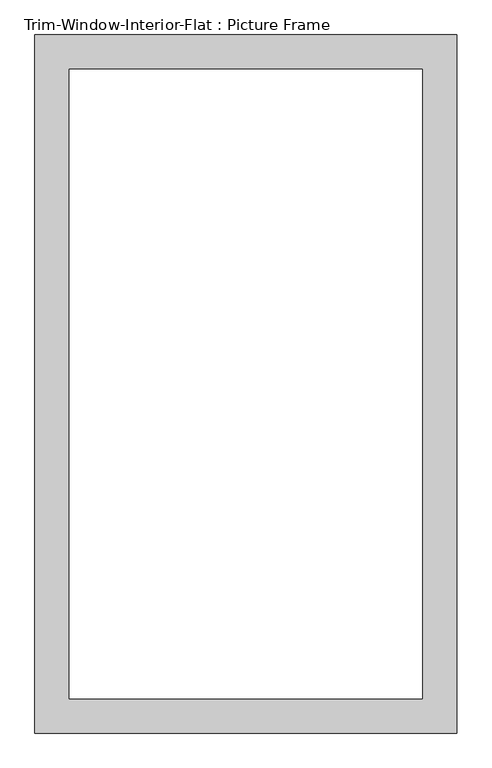
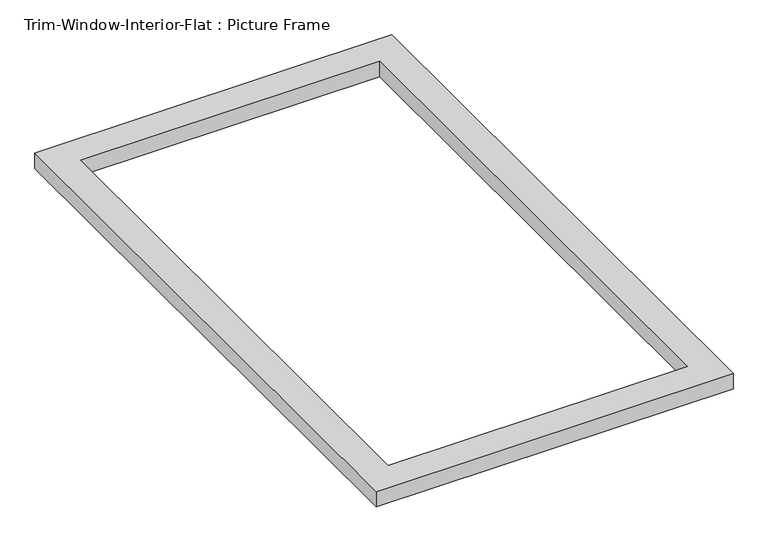
"""IFC4 building model written with IfcOpenShell, lengths in millimetres: proxy geometry, Trim-Window-Interior-Flat : Picture Frame."""

from ifc_helpers import new_model, si_unit, origin, origin_with_axes, place, context, project, spatial, polyline, outline, extrude, source, transform, mapped, element, save


def trim_window_interior_flat_picture_frame_e9fd5f45(model_context):
    return source(origin(), model_context, "Body", "SweptSolid", [
        extrude(outline(polyline([(349.25, 44.45), (349.25, -1111.25), (-349.25, -1111.25), (-349.25, 44.45), (349.25, 44.45)]), holes=[polyline([(292.1, -12.7), (-292.1, -12.7), (-292.1, -1054.1), (292.1, -1054.1), (292.1, -12.7)])]), origin_with_axes(), (0.0, 0.0, 1.0), 31.75),
    ])


if __name__ == "__main__":
    model = new_model("IFC4")
    model_context = context("Model", 3, world=origin())
    ifc_project = project(units=[si_unit("LENGTHUNIT", "METRE", prefix="MILLI")], contexts=[model_context])
    site = spatial("IfcSite", under=ifc_project)
    building = spatial("IfcBuilding", under=site)
    placement = place(None, origin())
    trim_window_interior_flat_picture_frame_shape = trim_window_interior_flat_picture_frame_e9fd5f45(model_context)
    element("IfcBuildingElementProxy", 1, Name="Trim-Window-Interior-Flat : Picture Frame", ObjectType="Trim-Window-Interior-Flat : Picture Frame", at=placement, inside=building, context=model_context, shape_type="MappedRepresentation", body=[
        mapped(trim_window_interior_flat_picture_frame_shape, transform((0.0, 0.0, 0.0), x_axis=(1.0, 0.0, 0.0), y_axis=(0.0, 1.0, 0.0), z_axis=(0.0, 0.0, 1.0))),
    ])
    save(model, "model.ifc")

# Revit data of these elements
# Type "Trim-Window-Interior-Flat : Picture Frame"
#   Trim Thickness_Picture Frame = 0' - 1 1/4"
#   Trim Width = 0' - 2 1/4"
#   Trim Thickness_with Sill = 0' - 0 3/4"
#   Sill Thickness = 0' - 1 1/4"
#   Opening Width [instance default] = 2' - 0"
#   Opening Height [instance default] = 3' - 0"
#   Default Elevation = 4' - 0"
#   Sill = no
#   Picture Frame = yes
#   Trim Material [instance default] = none
# Element 1 (IfcBuildingElementProxy, "Trim-Window-Interior-Flat : Picture Frame")
#   Opening Height = 3' - 6"
#   Trim Material = Wood - Stained
#   Materials on its faces: "Wood - Stained"
# Materials
#   "Wood - Stained": class "Wood", colour RGB 224 178 126, transparency 0, Cost = 0
